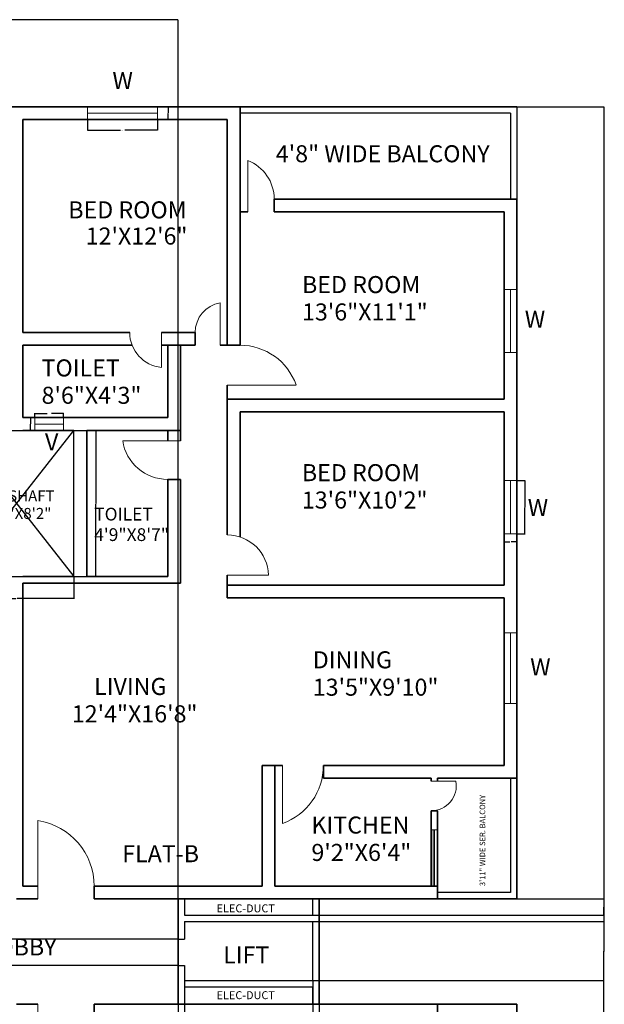
# Model space of a CAD drawing. Units: feet. Extents: x 5816 to 6644, y 25475 to 26788.
# Tile 23 of 23: x 6232 to 6644, y 26094 to 26788. Entities that reach past the tile are written whole.
import ezdxf

# ---------------------------------------------------------------- set-up
doc = ezdxf.new("R2010")
doc.units = ezdxf.units.FT
for name, color, linetype, lineweight in [('A-ANNO-DIMS', 2, 'Continuous', 13), ('A-ANNO-TEXT', 7, 'Continuous', 18), ('A-AREA-IDEN', 7, 'Continuous', 18), ('A-DOOR', 3, 'Continuous', 18), ('A-FLOR-EVTR', 4, 'Continuous', 25), ('A-FLOR-RAIL', 8, 'Continuous', 25), ('A-FLOR-SHFT', 8, 'Continuous', 25), ('A-GLAZ', 4, 'Continuous', 18), ('A-WALL', 7, 'Continuous', 35)]:
    doc.layers.add(name, color=color, linetype=linetype, lineweight=lineweight)
doc.styles.get("Standard").update_dxf_attribs({"font": 'arial.ttf'})
doc.dimstyles.get("Standard").update_dxf_attribs({"dimtxt": 0.18, "dimasz": 0.18, "dimexe": 0.18, "dimexo": 0.0625, "dimgap": 0.09, "dimtad": 0, "dimtih": 1, "dimtoh": 1, "dimdec": 4, "dimzin": 0, "dimdsep": 46, "dimtxsty": 'Standard', "dimcen": 0.09, "dimadec": 0, "dimazin": 0, "dimtfac": 1, "dimtdec": 4, "dimtofl": 0, "dimtmove": 0, "dimatfit": 3, "dimfxl": 1, "dimtolj": 1, "dimtzin": 0, "dimarcsym": 0})

# ---------------------------------------------------------------- blocks, each defined once
blk = doc.blocks.new('DOOR-BALCONY')
blk.add_line((0, 36.11), (0, 0))
blk.add_arc((10.54, 9), 29.09, 111.24329, 180)
blk = doc.blocks.new('DOOR-BEDROOM-INNER')
blk.add_line((0, 29.82), (0, 0))
blk.add_arc((-3.45, 9), 21.11, 0, 80.59123)
blk = doc.blocks.new('DOOR-BEDROOM-BALCONY')
blk.add_line((-48.41, 0), (0, 0))
blk.add_arc((-9, -13.73), 41.74, 90, 160.78776)
blk = doc.blocks.new('DOOR-BEDROOM-SIDE')
blk.add_line((-28.98, 0), (0, 0))
blk.add_arc((0.03, -0.75), 29.02, 90, 178.52212)
blk = doc.blocks.new('DOOR-KITCHEN')
blk.add_line((0, -40.87), (0, 0))
blk.add_arc((14.45, 0), 43.35, 180, 250.52864)
blk = doc.blocks.new('DOOR-SERVICE-BALCONY')
blk.add_line((-17.56, 0), (0, 0))
blk.add_arc((0, -2.91), 17.8, 170.58679, 270)
blk = doc.blocks.new('DOOR-FLAT-ENTRY')
blk.add_line((0, 55.13), (0, 0))
blk.add_arc((7.05, 9.01), 46.66, 98.693, 180)
blk = doc.blocks.new('DOOR-BATH-ENSUITE')
blk.add_line((0, -24.59), (0, 0))
blk.add_arc((-2.33, 0.02), 24.72, 275.40734, 0)
blk = doc.blocks.new('DOOR-BATH-HALL')
blk.add_line((40.72, 0), (0, 0))
blk.add_arc((9, 4.86), 32.09, 270, 351.28818)
blk = doc.blocks.new('WIN-DINING')
for p, q in [((0, 0), (9, 0)), ((4.5, 0), (4.5, -49.84)), ((0, -49.84), (9, -49.84))]:
    blk.add_line(p, q)
blk = doc.blocks.new('WIN-BEDROOM-SIDE')
for p, q in [((0, 0), (9, 0)), ((4.5, 0), (4.5, -37.54)), ((0, -37.54), (9, -37.54))]:
    blk.add_line(p, q)
blk = doc.blocks.new('WIN-BEDROOM-BALCONY')
for p, q in [((0, 0), (9, 0)), ((4.5, 0), (4.5, -44.28)), ((0, -44.28), (9, -44.28))]:
    blk.add_line(p, q)
blk = doc.blocks.new('WIN-BEDROOM-INNER')
for p, q in [((49.5, 0), (49.5, -9)), ((0, 0), (0, -9)), ((0, -4.5), (49.5, -4.5))]:
    blk.add_line(p, q)
blk = doc.blocks.new('WIN-KITCHEN')
for p, q in [((0, 0), (4.5, 0)), ((2, 0), (2, -39.61)), ((3, 0), (3, -39.61))]:
    blk.add_line(p, q)
blk = doc.blocks.new('WIN-VENT-NARROW')
for p, q in [((0, 0), (0, -9)), ((20.24, 0), (20.24, -9)), ((0, -4.5), (20.24, -4.5))]:
    blk.add_line(p, q)
blk = doc.blocks.new('VENT-SHAFT')
for p, q in [((0, 0), (0, 103)), ((0, 103), (81, 103)), ((0, 103), (81, 0)), ((0, 0), (81, 103)), ((81, 103), (45, 103)), ((81, 0), (81, 103)), ((0, 0), (81, 0)), ((81, 0), (45, 0))]:
    blk.add_line(p, q)
blk = doc.blocks.new('RAIL-BALCONY-CORNER')
for p, q in [((0, 0), (0, -65)), ((0, 0), (195, 0)), ((4.5, -4.5), (4.5, -65)), ((4.5, -4.5), (195, -4.5))]:
    blk.add_line(p, q)
blk = doc.blocks.new('*D39')
at = {"layer": 'A-ANNO-DIMS', "color": 0, "lineweight": -2, "transparency": 16777216}
for p, q in [((6582.37, 26463.28), (6588.12, 26463.28)), ((6587.94, 26463.1), (6587.94, 26444.69)), ((6587.94, 26425.92), (6587.94, 26444.33)), ((6582.37, 26425.74), (6588.12, 26425.74))]:
    blk.add_line(p, q, dxfattribs=at)
at = {"layer": 'A-ANNO-DIMS', "color": 0, "transparency": 16777216}
for points in [[(6587.91, 26463.1), (6587.97, 26463.1), (6587.94, 26463.28)], [(6587.91, 26425.92), (6587.97, 26425.92), (6587.94, 26425.74)]]:
    blk.add_solid(points, dxfattribs=at)
at = {"layer": 'Defpoints', "color": 0, "transparency": 16777216}
for p in [(6582.31, 26463.28), (6582.31, 26425.74), (6587.94, 26425.74)]:
    blk.add_point(p, dxfattribs=at)
at = {"layer": 'A-ANNO-DIMS', "color": 0, "transparency": 16777216, "insert": (6587.94, 26444.51), "char_height": 0.18, "attachment_point": 5}
blk.add_mtext('\\A1;SIDE BR WDW 38 TYP.', dxfattribs=at)
blk = doc.blocks.new('*D40')
at = {"layer": 'A-ANNO-DIMS', "color": 0, "lineweight": -2, "transparency": 16777216}
for p, q in [((6573.31, 26425.68), (6573.31, 26419.93)), ((6582.31, 26425.68), (6582.31, 26419.93)), ((6573.49, 26420.11), (6577.35, 26420.11)), ((6582.13, 26420.11), (6578.27, 26420.11))]:
    blk.add_line(p, q, dxfattribs=at)
at = {"layer": 'A-ANNO-DIMS', "color": 0, "transparency": 16777216}
for points in [[(6573.49, 26420.14), (6573.49, 26420.08), (6573.31, 26420.11)], [(6582.13, 26420.14), (6582.13, 26420.08), (6582.31, 26420.11)]]:
    blk.add_solid(points, dxfattribs=at)
at = {"layer": 'Defpoints', "color": 0, "transparency": 16777216}
for p in [(6573.31, 26425.74), (6582.31, 26425.74), (6573.31, 26420.11)]:
    blk.add_point(p, dxfattribs=at)
at = {"layer": 'A-ANNO-DIMS', "color": 0, "transparency": 16777216, "insert": (6577.81, 26420.11), "char_height": 0.18, "attachment_point": 5}
blk.add_mtext('\\A1;9 TYP.', dxfattribs=at)
blk = doc.blocks.new('*D43')
at = {"layer": 'A-ANNO-DIMS', "color": 0, "lineweight": -2, "transparency": 16777216}
for p, q in [((6279.74, 26717.52), (6279.74, 26709.98)), ((6329.24, 26717.52), (6329.24, 26709.98)), ((6279.92, 26710.16), (6302.97, 26710.16)), ((6329.06, 26710.16), (6306.01, 26710.16))]:
    blk.add_line(p, q, dxfattribs=at)
at = {"layer": 'A-ANNO-DIMS', "color": 0, "transparency": 16777216}
for points in [[(6279.92, 26710.19), (6279.92, 26710.13), (6279.74, 26710.16)], [(6329.06, 26710.19), (6329.06, 26710.13), (6329.24, 26710.16)]]:
    blk.add_solid(points, dxfattribs=at)
at = {"layer": 'Defpoints', "color": 0, "transparency": 16777216}
for p in [(6279.74, 26717.58), (6329.24, 26717.58), (6329.24, 26710.16)]:
    blk.add_point(p, dxfattribs=at)
at = {"layer": 'A-ANNO-DIMS', "color": 0, "transparency": 16777216, "insert": (6304.49, 26710.16), "char_height": 0.18, "attachment_point": 5}
blk.add_mtext('\\A1;INNER BR WDW 50 TYP.', dxfattribs=at)
blk = doc.blocks.new('*D44')
at = {"layer": 'A-ANNO-DIMS', "color": 0, "lineweight": -2, "transparency": 16777216}
for p, q in [((6329.31, 26726.58), (6336.85, 26726.58)), ((6336.67, 26726.4), (6336.67, 26722.27)), ((6329.31, 26717.58), (6336.85, 26717.58)), ((6336.67, 26717.76), (6336.67, 26721.9))]:
    blk.add_line(p, q, dxfattribs=at)
at = {"layer": 'A-ANNO-DIMS', "color": 0, "transparency": 16777216}
for points in [[(6336.64, 26726.4), (6336.7, 26726.4), (6336.67, 26726.58)], [(6336.64, 26717.76), (6336.7, 26717.76), (6336.67, 26717.58)]]:
    blk.add_solid(points, dxfattribs=at)
at = {"layer": 'Defpoints', "color": 0, "transparency": 16777216}
for p in [(6329.24, 26726.58), (6336.67, 26726.58), (6329.24, 26717.58)]:
    blk.add_point(p, dxfattribs=at)
at = {"layer": 'A-ANNO-DIMS', "color": 0, "transparency": 16777216, "insert": (6336.67, 26722.08), "char_height": 0.18, "attachment_point": 5}
blk.add_mtext('\\A1;9 TYP.', dxfattribs=at)
blk = doc.blocks.new('*D51')
at = {"layer": 'A-ANNO-DIMS', "color": 0, "lineweight": -2, "transparency": 16777216}
for p, q in [((6242.76, 26507.65), (6242.76, 26510.8)), ((6242.94, 26510.62), (6251.38, 26510.62)), ((6262.82, 26510.62), (6254.38, 26510.62)), ((6263, 26507.65), (6263, 26510.8))]:
    blk.add_line(p, q, dxfattribs=at)
at = {"layer": 'A-ANNO-DIMS', "color": 0, "transparency": 16777216}
for points in [[(6242.94, 26510.65), (6242.94, 26510.59), (6242.76, 26510.62)], [(6262.82, 26510.65), (6262.82, 26510.59), (6263, 26510.62)]]:
    blk.add_solid(points, dxfattribs=at)
at = {"layer": 'Defpoints', "color": 0, "transparency": 16777216}
for p in [(6263, 26510.62), (6242.76, 26507.58), (6263, 26507.58)]:
    blk.add_point(p, dxfattribs=at)
at = {"layer": 'A-ANNO-DIMS', "color": 0, "transparency": 16777216, "insert": (6252.88, 26510.62), "char_height": 0.18, "attachment_point": 5}
blk.add_mtext('\\A1;NARROW VENT 20 TYP.', dxfattribs=at)
blk = doc.blocks.new('*D52')
at = {"layer": 'A-ANNO-DIMS', "color": 0, "lineweight": -2, "transparency": 16777216}
for p, q in [((6242.7, 26507.58), (6239.54, 26507.58)), ((6239.72, 26507.4), (6239.72, 26503.27)), ((6239.72, 26498.76), (6239.72, 26502.9)), ((6242.7, 26498.58), (6239.54, 26498.58))]:
    blk.add_line(p, q, dxfattribs=at)
at = {"layer": 'A-ANNO-DIMS', "color": 0, "transparency": 16777216}
for points in [[(6239.69, 26507.4), (6239.75, 26507.4), (6239.72, 26507.58)], [(6239.69, 26498.76), (6239.75, 26498.76), (6239.72, 26498.58)]]:
    blk.add_solid(points, dxfattribs=at)
at = {"layer": 'Defpoints', "color": 0, "transparency": 16777216}
for p in [(6239.72, 26507.58), (6242.76, 26507.58), (6242.76, 26498.58)]:
    blk.add_point(p, dxfattribs=at)
at = {"layer": 'A-ANNO-DIMS', "color": 0, "transparency": 16777216, "insert": (6239.72, 26503.08), "char_height": 0.18, "attachment_point": 5}
blk.add_mtext('\\A1;9 TYP.', dxfattribs=at)
blk = doc.blocks.new('*D53')
at = {"layer": 'A-ANNO-DIMS', "color": 0, "lineweight": -2, "transparency": 16777216}
for p, q in [((6270.37, 26498.58), (6285.94, 26498.58)), ((6285.76, 26498.4), (6285.76, 26447.27)), ((6285.76, 26395.76), (6285.76, 26446.9)), ((6270.37, 26395.58), (6285.94, 26395.58))]:
    blk.add_line(p, q, dxfattribs=at)
at = {"layer": 'A-ANNO-DIMS', "color": 0, "transparency": 16777216}
for points in [[(6285.73, 26498.4), (6285.79, 26498.4), (6285.76, 26498.58)], [(6285.73, 26395.76), (6285.79, 26395.76), (6285.76, 26395.58)]]:
    blk.add_solid(points, dxfattribs=at)
at = {"layer": 'Defpoints', "color": 0, "transparency": 16777216}
for p in [(6270.31, 26498.58), (6285.76, 26498.58), (6270.31, 26395.58)]:
    blk.add_point(p, dxfattribs=at)
at = {"layer": 'A-ANNO-DIMS', "color": 0, "transparency": 16777216, "insert": (6285.76, 26447.08), "char_height": 0.18, "attachment_point": 5}
blk.add_mtext('\\A1;SHAFT 103 TYP.', dxfattribs=at)
blk = doc.blocks.new('*D54')
at = {"layer": 'A-ANNO-DIMS', "color": 0, "lineweight": -2, "transparency": 16777216}
for p, q in [((6189.31, 26395.52), (6189.31, 26379.95)), ((6270.31, 26395.52), (6270.31, 26379.95)), ((6189.49, 26380.13), (6229.28, 26380.13)), ((6270.13, 26380.13), (6230.34, 26380.13))]:
    blk.add_line(p, q, dxfattribs=at)
at = {"layer": 'A-ANNO-DIMS', "color": 0, "transparency": 16777216}
for points in [[(6189.49, 26380.16), (6189.49, 26380.1), (6189.31, 26380.13)], [(6270.13, 26380.16), (6270.13, 26380.1), (6270.31, 26380.13)]]:
    blk.add_solid(points, dxfattribs=at)
at = {"layer": 'Defpoints', "color": 0, "transparency": 16777216}
for p in [(6189.31, 26395.58), (6270.31, 26395.58), (6270.31, 26380.13)]:
    blk.add_point(p, dxfattribs=at)
at = {"layer": 'A-ANNO-DIMS', "color": 0, "transparency": 16777216, "insert": (6229.81, 26380.13), "char_height": 0.18, "attachment_point": 5}
blk.add_mtext('\\A1;81 TYP.', dxfattribs=at)
blk = doc.blocks.new('*D56')
at = {"layer": 'A-ANNO-DIMS', "color": 0, "lineweight": -2, "transparency": 16777216}
for p, q in [((6582.37, 26726.58), (6643.64, 26726.58)), ((6643.46, 26726.4), (6643.46, 26131.64)), ((6643.46, 25536.52), (6643.46, 26131.28)), ((6582.37, 25536.34), (6643.64, 25536.34))]:
    blk.add_line(p, q, dxfattribs=at)
at = {"layer": 'A-ANNO-DIMS', "color": 0, "transparency": 16777216}
for points in [[(6643.43, 26726.4), (6643.49, 26726.4), (6643.46, 26726.58)], [(6643.43, 25536.52), (6643.49, 25536.52), (6643.46, 25536.34)]]:
    blk.add_solid(points, dxfattribs=at)
at = {"layer": 'Defpoints', "color": 0, "transparency": 16777216}
for p in [(6582.31, 26726.58), (6643.46, 26726.58), (6582.31, 25536.34)]:
    blk.add_point(p, dxfattribs=at)
at = {"layer": 'A-ANNO-DIMS', "color": 0, "transparency": 16777216, "insert": (6643.46, 26131.46), "char_height": 0.18, "attachment_point": 5}
blk.add_mtext('\\A1;1190.2', dxfattribs=at)
blk = doc.blocks.new('*D59')
at = {"layer": 'A-ANNO-DIMS', "color": 0, "lineweight": -2, "transparency": 16777216}
for p, q in [((6343.68, 26168.52), (6343.68, 25475.01)), ((6442.98, 26168.59), (6442.98, 25475.01)), ((6343.86, 25475.19), (6393, 25475.19)), ((6442.8, 25475.19), (6393.65, 25475.19))]:
    blk.add_line(p, q, dxfattribs=at)
at = {"layer": 'A-ANNO-DIMS', "color": 0, "transparency": 16777216}
for points in [[(6343.86, 25475.22), (6343.86, 25475.16), (6343.68, 25475.19)], [(6442.8, 25475.22), (6442.8, 25475.16), (6442.98, 25475.19)]]:
    blk.add_solid(points, dxfattribs=at)
at = {"layer": 'Defpoints', "color": 0, "transparency": 16777216}
for p in [(6343.68, 26168.58), (6442.98, 26168.65), (6442.98, 25475.19)]:
    blk.add_point(p, dxfattribs=at)
at = {"layer": 'A-ANNO-DIMS', "color": 0, "transparency": 16777216, "insert": (6393.33, 25475.19), "char_height": 0.18, "attachment_point": 5}
blk.add_mtext('\\A1;99.3', dxfattribs=at)
blk = doc.blocks.new('*D60')
at = {"layer": 'A-ANNO-DIMS', "color": 0, "lineweight": -2, "transparency": 16777216}
for p, q in [((6106.98, 26094.4), (6106.98, 26787.91)), ((6107.16, 26787.73), (6224.93, 26787.73)), ((6343.5, 26787.73), (6225.72, 26787.73)), ((6343.68, 26094.4), (6343.68, 26787.91))]:
    blk.add_line(p, q, dxfattribs=at)
at = {"layer": 'A-ANNO-DIMS', "color": 0, "transparency": 16777216}
for points in [[(6107.16, 26787.76), (6107.16, 26787.7), (6106.98, 26787.73)], [(6343.5, 26787.76), (6343.5, 26787.7), (6343.68, 26787.73)]]:
    blk.add_solid(points, dxfattribs=at)
at = {"layer": 'Defpoints', "color": 0, "transparency": 16777216}
for p in [(6343.68, 26787.73), (6106.98, 26094.34), (6343.68, 26094.34)]:
    blk.add_point(p, dxfattribs=at)
at = {"layer": 'A-ANNO-DIMS', "color": 0, "transparency": 16777216, "insert": (6225.33, 26787.73), "char_height": 0.18, "attachment_point": 5}
blk.add_mtext('\\A1;236.7', dxfattribs=at)
blk = doc.blocks.new('*D69')
at = {"layer": 'A-ANNO-DIMS', "color": 0, "lineweight": -2, "transparency": 16777216}
for p, q in [((6438.54, 26152.62), (6643.64, 26152.62)), ((6643.46, 26152.44), (6643.46, 26132.06)), ((6643.46, 26111.31), (6643.46, 26131.69)), ((6438.54, 26111.13), (6643.64, 26111.13))]:
    blk.add_line(p, q, dxfattribs=at)
at = {"layer": 'A-ANNO-DIMS', "color": 0, "transparency": 16777216}
for points in [[(6643.43, 26152.44), (6643.49, 26152.44), (6643.46, 26152.62)], [(6643.43, 26111.31), (6643.49, 26111.31), (6643.46, 26111.13)]]:
    blk.add_solid(points, dxfattribs=at)
at = {"layer": 'Defpoints', "color": 0, "transparency": 16777216}
for p in [(6438.48, 26152.62), (6643.46, 26152.62), (6438.48, 26111.13)]:
    blk.add_point(p, dxfattribs=at)
at = {"layer": 'A-ANNO-DIMS', "color": 0, "transparency": 16777216, "insert": (6643.46, 26131.88), "char_height": 0.18, "attachment_point": 5}
blk.add_mtext('\\A1;41.49', dxfattribs=at)
blk = doc.blocks.new('*D70')
at = {"layer": 'A-ANNO-DIMS', "color": 0, "lineweight": -2, "transparency": 16777216}
for p, q in [((6348.24, 26168.58), (6643.64, 26168.58)), ((6643.46, 26168.4), (6643.46, 26163.04)), ((6643.46, 26157.3), (6643.46, 26162.67)), ((6348.24, 26157.12), (6643.64, 26157.12))]:
    blk.add_line(p, q, dxfattribs=at)
at = {"layer": 'A-ANNO-DIMS', "color": 0, "transparency": 16777216}
for points in [[(6643.43, 26168.4), (6643.49, 26168.4), (6643.46, 26168.58)], [(6643.43, 26157.3), (6643.49, 26157.3), (6643.46, 26157.12)]]:
    blk.add_solid(points, dxfattribs=at)
at = {"layer": 'Defpoints', "color": 0, "transparency": 16777216}
for p in [(6348.18, 26168.58), (6643.46, 26168.58), (6348.18, 26157.12)]:
    blk.add_point(p, dxfattribs=at)
at = {"layer": 'A-ANNO-DIMS', "color": 0, "transparency": 16777216, "insert": (6643.46, 26162.85), "char_height": 0.18, "attachment_point": 5}
blk.add_mtext('\\A1;11.462', dxfattribs=at)
blk = doc.blocks.new('*D71')
at = {"layer": 'A-ANNO-DIMS', "color": 0, "lineweight": -2, "transparency": 16777216}
for p, q in [((6343.61, 26140.22), (5815.98, 26140.22)), ((5816.16, 26140.04), (5816.16, 26131.1)), ((5816.16, 26121.79), (5816.16, 26130.74)), ((6343.61, 26121.61), (5815.98, 26121.61))]:
    blk.add_line(p, q, dxfattribs=at)
at = {"layer": 'A-ANNO-DIMS', "color": 0, "transparency": 16777216}
for points in [[(5816.13, 26140.04), (5816.19, 26140.04), (5816.16, 26140.22)], [(5816.13, 26121.79), (5816.19, 26121.79), (5816.16, 26121.61)]]:
    blk.add_solid(points, dxfattribs=at)
at = {"layer": 'Defpoints', "color": 0, "transparency": 16777216}
for p in [(6343.68, 26140.22), (5816.16, 26121.61), (6343.68, 26121.61)]:
    blk.add_point(p, dxfattribs=at)
at = {"layer": 'A-ANNO-DIMS', "color": 0, "transparency": 16777216, "insert": (5816.16, 26130.92), "char_height": 0.18, "attachment_point": 5}
blk.add_mtext('\\A1;18.61', dxfattribs=at)
blk = doc.blocks.new('*D73')
at = {"layer": 'A-ANNO-DIMS', "color": 0, "lineweight": -2, "transparency": 16777216}
for p, q in [((6348.18, 26111.07), (6348.18, 25475.01)), ((6438.48, 26111.07), (6438.48, 25475.01)), ((6348.36, 25475.19), (6393, 25475.19)), ((6438.3, 25475.19), (6393.65, 25475.19))]:
    blk.add_line(p, q, dxfattribs=at)
at = {"layer": 'A-ANNO-DIMS', "color": 0, "transparency": 16777216}
for points in [[(6348.36, 25475.22), (6348.36, 25475.16), (6348.18, 25475.19)], [(6438.3, 25475.22), (6438.3, 25475.16), (6438.48, 25475.19)]]:
    blk.add_solid(points, dxfattribs=at)
at = {"layer": 'Defpoints', "color": 0, "transparency": 16777216}
for p in [(6348.18, 26111.13), (6438.48, 26111.13), (6438.48, 25475.19)]:
    blk.add_point(p, dxfattribs=at)
at = {"layer": 'A-ANNO-DIMS', "color": 0, "transparency": 16777216, "insert": (6393.33, 25475.19), "char_height": 0.18, "attachment_point": 5}
blk.add_mtext('\\A1;90.3', dxfattribs=at)

msp = doc.modelspace()

# ---------------------------------------------------------------- linework, layer by layer
at = {"layer": 'A-FLOR-EVTR'}
for p, q in [((6343.6763, 26168.5846), (6343.6763, 26140.2241)), ((6348.1763, 26152.6231), (6438.4781, 26152.6231)), ((6348.1763, 26152.6231), (6348.1763, 26140.2241)), ((6438.4781, 26111.129), (6438.4781, 26152.6231)), ((6343.6763, 26140.2241), (6348.1763, 26140.2241)), ((6343.6763, 26121.6124), (6348.1763, 26121.6124)), ((6343.6763, 26121.6124), (6343.6763, 26094.3368)), ((6348.1763, 26121.6124), (6348.1763, 26111.129)), ((6348.1763, 26111.129), (6438.4781, 26111.129))]:
    msp.add_line(p, q, dxfattribs=at)
at = {"layer": 'A-FLOR-RAIL'}
msp.add_lwpolyline([(6577.8119, 26253.5846), (6577.8119, 26173.0846), (6526.3119, 26173.0846)], dxfattribs=at)
at = {"layer": 'A-FLOR-SHFT'}
for p, q in [((6348.1763, 26168.5846), (6348.1763, 26157.1231)), ((6438.4781, 26157.1231), (6438.4781, 26168.6509)), ((6348.1763, 26157.1231), (6438.4781, 26157.1231)), ((6348.1763, 26106.629), (6438.4781, 26106.629)), ((6348.1763, 26106.629), (6348.1763, 26094.3368)), ((6438.4781, 26094.6509), (6438.4781, 26106.629))]:
    msp.add_line(p, q, dxfattribs=at)
at = {"layer": 'A-WALL'}
for p, q in [((5877.3119, 26726.5846), (6279.7398, 26726.5846)), ((6582.3119, 26726.5846), (6234.3119, 26726.5846)), ((6387.3119, 26661.5846), (6387.3119, 26726.5846)), ((6378.3119, 26717.5846), (6234.3119, 26717.5846)), ((6234.3119, 26717.5846), (6234.3119, 26567.5846)), ((6378.3119, 26661.5846), (6378.3119, 26717.5846)), ((6378.3119, 26558.5846), (6378.3119, 26668.7645)), ((6387.3119, 26558.5846), (6387.3119, 26668.7645)), ((6582.3119, 26661.5846), (6411.3119, 26661.5846)), ((6411.3119, 26652.5846), (6411.3119, 26661.5846)), ((6582.3119, 26661.5846), (6582.3119, 26652.5846)), ((6392.7622, 26652.5846), (6387.3119, 26652.5846)), ((6573.3119, 26652.5846), (6411.3119, 26652.5846)), ((6573.3119, 26652.5846), (6573.3119, 26520.5846)), ((6582.3119, 26652.5846), (6582.3119, 26253.5846)), ((6234.3119, 26567.5846), (6309.5426, 26567.5846)), ((6331.936, 26567.5846), (6355.6538, 26567.5846)), ((6355.6538, 26567.5846), (6355.6538, 26558.5846)), ((6234.3119, 26558.5846), (6311.248, 26558.5846)), ((6234.3119, 26558.5846), (6311.248, 26558.5846)), ((6234.3119, 26507.5846), (6234.3119, 26558.5846)), ((6331.936, 26558.5846), (6355.6538, 26558.5846)), ((6331.936, 26558.5846), (6336.3119, 26558.5846)), ((6336.3119, 26558.5846), (6336.3119, 26507.5846)), ((6345.3119, 26558.5846), (6345.3119, 26491.3288)), ((6373.3112, 26558.5846), (6387.3119, 26558.5846)), ((6378.3119, 26520.5846), (6378.3119, 26530.5827)), ((6378.3119, 26530.5827), (6378.3119, 26424.9443)), ((6573.3119, 26520.5846), (6378.3119, 26520.5846)), ((6573.3119, 26511.5846), (6387.3119, 26511.5846)), ((6387.3119, 26511.5846), (6387.3119, 26423.5033)), ((6573.3119, 26511.5846), (6573.3119, 26389.5846)), ((6582.3119, 26511.5846), (6582.3119, 26253.5846)), ((6336.3119, 26507.5846), (6234.3119, 26507.5846)), ((6345.3119, 26498.5846), (6279.3119, 26498.5846)), ((6279.3119, 26395.5846), (6279.3119, 26498.5846)), ((6336.3119, 26498.5846), (6336.3119, 26491.3288)), ((6336.3119, 26464.0978), (6336.3119, 26395.5846)), ((6336.3119, 26464.0978), (6345.3119, 26464.0978)), ((6345.3119, 26464.0978), (6345.3119, 26391.0846)), ((6336.3119, 26391.0846), (6234.3119, 26391.0846)), ((6234.3119, 26391.0846), (6234.3119, 26177.5846)), ((6336.3119, 26395.5846), (6279.3119, 26395.5846)), ((6336.3119, 26391.0846), (6345.3119, 26391.0846)), ((6378.3119, 26396.677), (6378.3119, 26380.5846)), ((6573.3119, 26389.5846), (6378.3119, 26389.5846)), ((6573.3119, 26380.5846), (6378.3119, 26380.5846)), ((6573.3119, 26380.5846), (6573.3119, 26262.5846)), ((6582.3119, 26380.5846), (6582.3119, 26262.5846)), ((6417.0917, 26262.5846), (6402.8119, 26262.5846)), ((6402.8119, 26253.5846), (6402.8119, 26262.5846)), ((6411.8119, 26177.5846), (6411.8119, 26262.5846)), ((6573.3119, 26262.5846), (6445.9911, 26262.5846)), ((6445.9911, 26262.5846), (6445.9911, 26253.5846)), ((6582.3119, 26262.5846), (6582.3119, 26168.5846)), ((6402.8119, 26177.5846), (6402.8119, 26253.5846)), ((6521.8119, 26253.5846), (6445.9911, 26253.5846)), ((6521.8119, 26253.5846), (6521.8119, 26251.4059)), ((6573.3119, 26253.5846), (6526.3119, 26253.5846)), ((6526.3119, 26253.5846), (6526.3119, 26251.4059)), ((6573.3119, 26253.5846), (6582.3119, 26253.5846)), ((6521.8119, 26230.6968), (6521.8119, 26177.5846)), ((6526.3119, 26230.6968), (6521.8119, 26230.6968)), ((6526.3119, 26230.6968), (6526.3119, 26168.5846)), ((6244.9332, 26177.5846), (6234.3119, 26177.5846)), ((6284.5408, 26177.5916), (6284.5408, 26168.5846)), ((6402.8119, 26177.5846), (6284.5408, 26177.5846)), ((6526.3119, 26177.5846), (6411.8119, 26177.5846)), ((6244.9332, 26168.5846), (6229.8119, 26168.5846)), ((6582.3119, 26168.5846), (6284.5408, 26168.5846)), ((6442.9781, 26094.6509), (6442.9781, 26168.6509)), ((6244.9332, 26094.3368), (6229.8119, 26094.3368)), ((6582.3119, 26094.3368), (6284.5408, 26094.3368)), ((6284.5408, 26085.3298), (6284.5408, 26094.3368)), ((6526.3119, 26032.2246), (6526.3119, 26094.3368)), ((6582.3119, 26000.3368), (6582.3119, 26094.3368))]:
    msp.add_line(p, q, dxfattribs=at)

# ---------------------------------------------------------------- block references
at = {"layer": 'A-DOOR', "extrusion": (0, 0, -1), "zscale": -1}
for name, p in [('DOOR-BALCONY', (-6392.7622, 26652.5846)), ('DOOR-BEDROOM-INNER', (-6373.3112, 26558.5846)), ('DOOR-BATH-ENSUITE', (-6331.936, 26567.5846)), ('DOOR-BEDROOM-BALCONY', (-6378.3119, 26530.5827)), ('DOOR-BATH-HALL', (-6345.3119, 26491.3288)), ('DOOR-BEDROOM-SIDE', (-6378.3119, 26396.677)), ('DOOR-KITCHEN', (-6417.0917, 26262.5846)), ('DOOR-SERVICE-BALCONY', (-6521.8119, 26251.4059)), ('DOOR-FLAT-ENTRY', (-6244.9332, 26168.5846))]:
    msp.add_blockref(name, p, dxfattribs=at)
at = {"layer": 'A-DOOR', "rotation": 180}
msp.add_blockref('DOOR-FLAT-ENTRY', (6244.9332, 26094.3368), dxfattribs=at)
at = {"layer": 'A-FLOR-RAIL', "extrusion": (0, 0, -1), "zscale": -1}
msp.add_blockref('RAIL-BALCONY-CORNER', (-6582.3119, 26726.5846), dxfattribs=at)
at = {"layer": 'A-FLOR-SHFT'}
msp.add_blockref('VENT-SHAFT', (6189.3119, 26395.5846), dxfattribs=at)
at = {"layer": 'A-GLAZ'}
for name, p in [('WIN-BEDROOM-INNER', (6279.7398, 26726.5846)), ('WIN-BEDROOM-BALCONY', (6573.3119, 26597.7938)), ('WIN-VENT-NARROW', (6242.7596, 26507.5846)), ('WIN-DINING', (6573.3119, 26355.98))]:
    msp.add_blockref(name, p, dxfattribs=at)
at = {"layer": 'A-GLAZ', "rotation": 180}
msp.add_blockref('WIN-BEDROOM-SIDE', (6582.3119, 26425.7418), dxfattribs=at)
at = {"layer": 'A-GLAZ', "extrusion": (0, 0, -1), "zscale": -1}
msp.add_blockref('WIN-KITCHEN', (-6526.3119, 26217.1904), dxfattribs=at)

# ---------------------------------------------------------------- texts
at = {"layer": 'A-ANNO-DIMS'}
for s, height, p in [('12\'X12\'6"', 12, (6278.5712, 26629.5209)), ('13\'6"X11\'1"', 12, (6430.9226, 26576.0431)), ('8\'6"X4\'3"', 12, (6247.4686, 26517.3427)), ('13\'6"X10\'2"', 12, (6430.8066, 26443.5614)), ('6\'7"X8\'2"', 7.77416, (6208.7805, 26436.2088)), ('4\'9"X8\'7"', 8.98988, (6284.5435, 26420.686)), ('13\'5"X9\'10"', 12, (6438.5021, 26311.7189)), ('12\'4"X16\'8"', 12, (6268.7679, 26292.9516)), ('9\'2"X6\'4"', 12, (6437.5373, 26195.3316))]:
    msp.add_text(s, height=height, dxfattribs=at).set_placement(p)
at = {"layer": 'A-ANNO-TEXT'}
for s, p in [('W', (6297.3974, 26738.9938)), ('W', (6587.8398, 26570.8943)), ('V', (6249.8631, 26484.5411)), ('W', (6589.9222, 26438.374)), ('W', (6591.6371, 26325.9996))]:
    msp.add_text(s, height=12, dxfattribs=at).set_placement(p)
at = {"layer": 'A-AREA-IDEN'}
for s, height, p in [('4\'8" WIDE BALCONY', 12, (6412.4604, 26687.4804)), ('BED ROOM', 12, (6266.28, 26647.9509)), ('BED ROOM', 12, (6430.9226, 26595.32)), ('TOILET', 12, (6247.4686, 26536.6196)), ('BED ROOM', 12, (6430.8066, 26462.8383)), ('VENT SHAFT', 7.77416, (6195.225, 26448.5899)), ('TOILET', 8.98988, (6284.5435, 26435.1275)), ('DINING', 12, (6438.5021, 26330.9959)), ('LIVING', 12, (6284.4576, 26312.2285)), ('KITCHEN', 12, (6437.5373, 26214.6086)), ('FLAT-B', 12, (6304.2633, 26194.4287)), ('ELEC-DUCT', 5.61284, (6370.7969, 26159.1323)), ('LOBBY', 12, (6206.7608, 26128.7481)), ('LIFT', 12, (6375.3756, 26123.1576)), ('ELEC-DUCT', 5.61284, (6370.7969, 26097.9572))]:
    msp.add_text(s, height=height, dxfattribs=at).set_placement(p)
msp.add_text('3\'11" WIDE SER. BALCONY', height=3.901456, rotation=90, dxfattribs=at).set_placement((6559.9339, 26177.6201))

# ---------------------------------------------------------------- dimensions: what is measured, and where the dimension line sits
at = {"layer": 'A-ANNO-DIMS'}
for base, p1, p2, picture, middle in [((6343.6763, 26787.7346), (6106.9781, 26094.3368), (6343.6763, 26094.3368), '*D60', (6225.3272, 26787.7346)), ((6442.9781, 25475.1868), (6343.6763, 26168.5846), (6442.9781, 26168.6509), '*D59', (6393.3272, 25475.1868)), ((6438.4781, 25475.1868), (6348.1763, 26111.129), (6438.4781, 26111.129), '*D73', (6393.3272, 25475.1868))]:
    dim = msp.add_linear_dim(base=base, p1=p1, p2=p2, dimstyle='Standard', override={"dimdec": 1, "dimlfac": 1, "dimrnd": 0, "dimzin": 0, "dimdsep": 46, "dimlunit": 2}, dxfattribs=at)
    dim.commit()
    dim.dimension.update_dxf_attribs({"geometry": picture, "text_midpoint": middle})
for base, p1, p2, angle, text, picture, middle in [((6336.6683, 26726.5846), (6329.2428, 26717.5846), (6329.2428, 26726.5846), 90, '<> TYP.', '*D44', (6336.6683, 26722.0846)), ((6239.7243, 26507.5846), (6242.7596, 26498.5846), (6242.7596, 26507.5846), 90, '<> TYP.', '*D52', (6239.7243, 26503.0846)), ((6285.7619, 26498.5846), (6270.3119, 26395.5846), (6270.3119, 26498.5846), 90, 'SHAFT <> TYP.', '*D53', (6285.7619, 26447.0846)), ((6587.9423, 26425.7418), (6582.3119, 26463.2783), (6582.3119, 26425.7418), 270, 'SIDE BR WDW <> TYP.', '*D39', (6587.9423, 26444.51)), ((6573.3119, 26420.1113), (6582.3119, 26425.7418), (6573.3119, 26425.7418), 180, '<> TYP.', '*D40', (6577.8119, 26420.1113))]:
    dim = msp.add_linear_dim(base=base, p1=p1, p2=p2, angle=angle, text=text, dimstyle='Standard', override={"dimdec": 0, "dimlfac": 1, "dimrnd": 0, "dimzin": 0, "dimdsep": 46, "dimlunit": 2}, dxfattribs=at)
    dim.commit()
    dim.dimension.update_dxf_attribs({"geometry": picture, "text_midpoint": middle})
for base, p1, p2, override, picture, middle in [((6643.4619, 26726.5846), (6582.3119, 25536.3368), (6582.3119, 26726.5846), {"dimdec": 1, "dimlfac": 1, "dimrnd": 0, "dimzin": 0, "dimdsep": 46, "dimlunit": 2}, '*D56', (6643.4619, 26131.4607)), ((6643.46185, 26168.58464), (6348.17633, 26157.12305), (6348.17633, 26168.58464), {"dimdec": 3, "dimlfac": 1, "dimrnd": 0, "dimzin": 0, "dimdsep": 46, "dimlunit": 2}, '*D70', (6643.46185, 26162.85385)), ((6643.4619, 26152.6231), (6438.4781, 26111.129), (6438.4781, 26152.6231), {"dimdec": 2, "dimlfac": 1, "dimrnd": 0, "dimzin": 0, "dimdsep": 46, "dimlunit": 2}, '*D69', (6643.4619, 26131.876)), ((5816.1619, 26121.6124), (6343.6763, 26140.2241), (6343.6763, 26121.6124), {"dimdec": 2, "dimlfac": 1, "dimrnd": 0, "dimzin": 0, "dimdsep": 46, "dimlunit": 2}, '*D71', (5816.1619, 26130.9183))]:
    dim = msp.add_linear_dim(base=base, p1=p1, p2=p2, angle=90, dimstyle='Standard', override=override, dxfattribs=at)
    dim.commit()
    dim.dimension.update_dxf_attribs({"geometry": picture, "text_midpoint": middle})
for base, p1, p2, text, picture, middle in [((6329.2428, 26710.1592), (6279.7398, 26717.5846), (6329.2428, 26717.5846), 'INNER BR WDW <> TYP.', '*D43', (6304.4913, 26710.1592)), ((6262.9952, 26510.62), (6242.7596, 26507.5846), (6262.9952, 26507.5846), 'NARROW VENT <> TYP.', '*D51', (6252.8774, 26510.62)), ((6270.3119, 26380.1346), (6189.3119, 26395.5846), (6270.3119, 26395.5846), '<> TYP.', '*D54', (6229.8119, 26380.1346))]:
    dim = msp.add_linear_dim(base=base, p1=p1, p2=p2, text=text, dimstyle='Standard', override={"dimdec": 0, "dimlfac": 1, "dimrnd": 0, "dimzin": 0, "dimdsep": 46, "dimlunit": 2}, dxfattribs=at)
    dim.commit()
    dim.dimension.update_dxf_attribs({"geometry": picture, "text_midpoint": middle})

doc.saveas('drawing.dxf')
